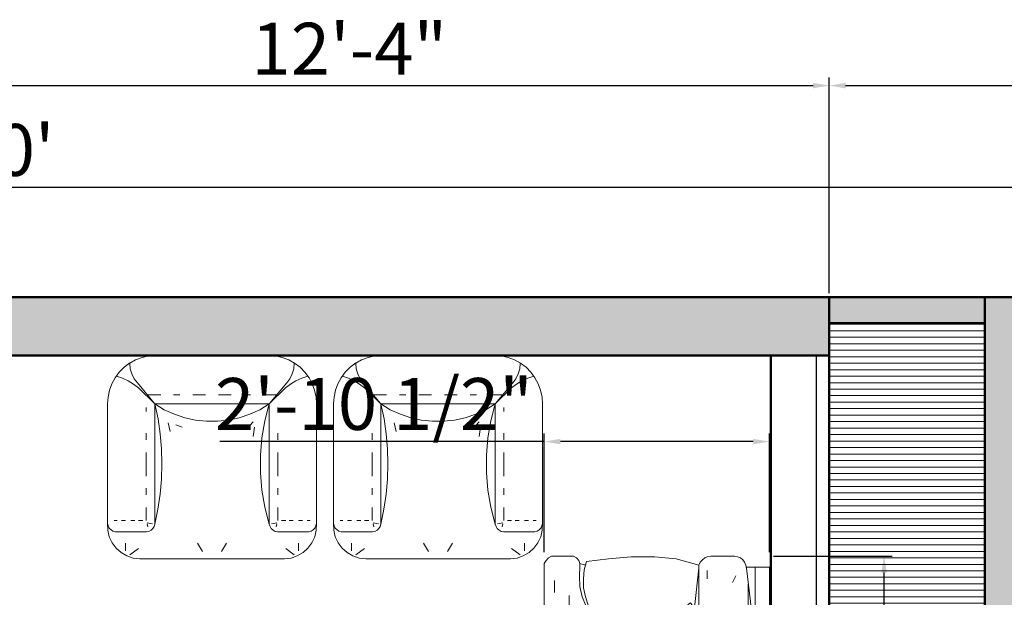
# Model space of a CAD drawing. Units: inches. Extents: x 1770 to 3141, y 984 to 1614.
# Tile 8 of 12: x 2115 to 2267, y 1519 to 1608. Entities that reach past the tile are written whole.
import ezdxf

# ---------------------------------------------------------------- set-up
doc = ezdxf.new("R2010")
doc.units = ezdxf.units.IN
for name, color, linetype, lineweight in [('A-ANNO-DIMS', 2, 'Continuous', 18), ('A-FLOR-PATT', 252, 'Continuous', 13), ('A-FURN', 8, 'Continuous', 18), ('A-GLAZ', 5, 'Continuous', 25), ('A-WALL', 7, 'Continuous', 50), ('A-WALL-PATT', 8, 'Continuous', 13)]:
    doc.layers.add(name, color=color, linetype=linetype, lineweight=lineweight)
doc.styles.get("Standard").update_dxf_attribs({"font": 'arial.ttf'})
doc.dimstyles.new('ISO-25', dxfattribs={"dimtxt": 8, "dimasz": 2.5, "dimexe": 1.25, "dimexo": 0.625, "dimtad": 1, "dimdec": 1, "dimlunit": 3, "dimtxsty": 'Standard', "dimcen": 2.5, "dimclrt": 1, "dimadec": 0, "dimazin": 0, "dimtfac": 1, "dimtdec": 1, "dimtmove": 0, "dimatfit": 3, "dimfxl": 1, "dimarcsym": 0})

# ---------------------------------------------------------------- blocks, each defined once
blk = doc.blocks.new('*D17')
at = {"layer": 'A-ANNO-DIMS', "color": 0, "lineweight": -2, "transparency": 16777216}
for p, q in [((1812.73, 1565.8), (1812.73, 1583.37)), ((2412.73, 1565.8), (2412.73, 1583.37)), ((1815.23, 1582.12), (2410.23, 1582.12))]:
    blk.add_line(p, q, dxfattribs=at)
at = {"layer": 'A-ANNO-DIMS', "color": 0, "transparency": 16777216}
for points in [[(1815.23, 1582.54), (1815.23, 1581.7), (1812.73, 1582.12)], [(2410.23, 1582.54), (2410.23, 1581.7), (2412.73, 1582.12)]]:
    blk.add_solid(points, dxfattribs=at)
at = {"layer": 'Defpoints', "color": 0, "transparency": 16777216}
for p in [(2412.73, 1582.12), (1812.73, 1565.18), (2412.73, 1565.18)]:
    blk.add_point(p, dxfattribs=at)
at = {"layer": 'A-ANNO-DIMS', "color": 0, "transparency": 16777216, "insert": (2112.73, 1586.83), "char_height": 8, "attachment_point": 5}
blk.add_mtext("50'", dxfattribs=at)
blk = doc.blocks.new('sofa-42')
at = {"color": 0, "linetype": 'ByBlock'}
for p, q in [((-0.038, 0.929), (-0.045, 0.917)), ((-0.045, 0.917), (-0.038, 0.929)), ((-0.045, 0.917), (-0.045, 0.824)), ((-0.045, 0.917), (-0.045, 0.824)), ((-0.028, 0.939), (-0.038, 0.929)), ((-0.038, 0.929), (-0.028, 0.939)), ((-0.015, 0.947), (-0.028, 0.939)), ((-0.028, 0.939), (-0.015, 0.947)), ((-0.003, 0.947), (-0.015, 0.947)), ((-0.015, 0.947), (-0.003, 0.947)), ((0.665, 0.947), (-0.003, 0.947)), ((-0.003, 0.947), (0.665, 0.947)), ((0.687, 0.942), (0.665, 0.947)), ((0.687, 0.942), (0.665, 0.947)), ((0.712, 0.932), (0.687, 0.942)), ((0.712, 0.932), (0.687, 0.942)), ((0.73, 0.917), (0.712, 0.932)), ((0.73, 0.917), (0.712, 0.932)), ((0.745, 0.897), (0.73, 0.917)), ((0.745, 0.897), (0.73, 0.917)), ((0.785, 0.917), (0.77, 0.897)), ((0.77, 0.897), (0.785, 0.917)), ((0.802, 0.932), (0.785, 0.917)), ((0.785, 0.917), (0.802, 0.932)), ((0.827, 0.942), (0.802, 0.932)), ((0.802, 0.932), (0.827, 0.942)), ((0.85, 0.947), (0.827, 0.942)), ((0.827, 0.942), (0.85, 0.947)), ((1.462, 0.947), (0.85, 0.947)), ((0.85, 0.947), (1.462, 0.947)), ((1.484, 0.942), (1.462, 0.947)), ((1.484, 0.942), (1.462, 0.947)), ((1.509, 0.932), (1.484, 0.942)), ((1.509, 0.932), (1.484, 0.942)), ((1.527, 0.917), (1.509, 0.932)), ((1.527, 0.917), (1.509, 0.932)), ((1.542, 0.897), (1.527, 0.917)), ((1.542, 0.897), (1.527, 0.917)), ((1.567, 0.897), (1.582, 0.917)), ((1.582, 0.917), (1.567, 0.897)), ((1.582, 0.917), (1.599, 0.932)), ((1.599, 0.932), (1.582, 0.917)), ((1.599, 0.932), (1.624, 0.942)), ((1.624, 0.942), (1.599, 0.932)), ((1.624, 0.942), (1.647, 0.947)), ((1.647, 0.947), (1.624, 0.942)), ((1.647, 0.947), (2.272, 0.947)), ((2.272, 0.947), (1.647, 0.947)), ((2.297, 0.942), (2.272, 0.947)), ((2.297, 0.942), (2.272, 0.947)), ((2.319, 0.932), (2.297, 0.942)), ((2.319, 0.932), (2.297, 0.942)), ((2.337, 0.917), (2.319, 0.932)), ((2.337, 0.917), (2.319, 0.932)), ((2.352, 0.897), (2.337, 0.917)), ((2.352, 0.897), (2.337, 0.917)), ((2.392, 0.917), (2.377, 0.897)), ((2.377, 0.897), (2.392, 0.917)), ((2.412, 0.932), (2.392, 0.917)), ((2.392, 0.917), (2.412, 0.932)), ((2.434, 0.942), (2.412, 0.932)), ((2.412, 0.932), (2.434, 0.942)), ((2.457, 0.947), (2.434, 0.942)), ((2.434, 0.942), (2.457, 0.947)), ((3.127, 0.947), (2.457, 0.947)), ((2.457, 0.947), (3.127, 0.947)), ((3.139, 0.947), (3.127, 0.947)), ((3.139, 0.947), (3.127, 0.947)), ((3.152, 0.939), (3.139, 0.947)), ((3.152, 0.939), (3.139, 0.947)), ((3.162, 0.929), (3.152, 0.939)), ((3.162, 0.929), (3.152, 0.939)), ((3.169, 0.917), (3.162, 0.929)), ((3.169, 0.917), (3.162, 0.929)), ((3.169, 0.824), (3.169, 0.917)), ((3.169, 0.917), (3.169, 0.824)), ((0.042, 0.909), (0.087, 0.889)), ((0.672, 0.892), (0.627, 0.849)), ((0.7, 0.874), (0.685, 0.824)), ((0.755, 0.872), (0.745, 0.897)), ((0.755, 0.872), (0.745, 0.897)), ((0.757, 0.849), (0.755, 0.872)), ((0.757, 0.849), (0.755, 0.872)), ((0.76, 0.872), (0.757, 0.849)), ((0.757, 0.849), (0.76, 0.872)), ((0.77, 0.897), (0.76, 0.872)), ((0.76, 0.872), (0.77, 0.897)), ((0.815, 0.874), (0.83, 0.824)), ((0.842, 0.892), (0.887, 0.849)), ((1.469, 0.892), (1.424, 0.849)), ((1.497, 0.874), (1.482, 0.824)), ((1.552, 0.872), (1.542, 0.897)), ((1.552, 0.872), (1.542, 0.897)), ((1.554, 0.849), (1.552, 0.872)), ((1.554, 0.849), (1.552, 0.872)), ((1.554, 0.849), (1.557, 0.872)), ((1.557, 0.872), (1.554, 0.849)), ((1.557, 0.872), (1.567, 0.897)), ((1.567, 0.897), (1.557, 0.872)), ((1.612, 0.874), (1.627, 0.824)), ((1.639, 0.892), (1.684, 0.849)), ((2.252, 0.887), (2.204, 0.877)), ((2.294, 0.884), (2.257, 0.829)), ((2.362, 0.872), (2.352, 0.897)), ((2.362, 0.872), (2.352, 0.897)), ((2.364, 0.849), (2.362, 0.872)), ((2.364, 0.849), (2.362, 0.872)), ((2.367, 0.872), (2.364, 0.849)), ((2.364, 0.849), (2.367, 0.872)), ((2.377, 0.897), (2.367, 0.872)), ((2.367, 0.872), (2.377, 0.897)), ((2.437, 0.884), (2.474, 0.829)), ((2.477, 0.887), (2.477, 0.877)), ((3.067, 0.904), (3.017, 0.904)), ((0.04, 0.799), (0.037, 0.839)), ((0.757, 0.345), (0.757, 0.849)), ((1.554, 0.06), (1.554, 0.849)), ((2.364, 0.345), (2.364, 0.849)), ((3.004, 0.842), (2.929, 0.842)), ((-0.045, 0.824), (-0.038, 0.812)), ((-0.045, 0.824), (-0.038, 0.812)), ((-0.038, 0.812), (-0.028, 0.802)), ((-0.038, 0.812), (-0.028, 0.802)), ((-0.028, 0.802), (-0.015, 0.797)), ((-0.028, 0.802), (-0.015, 0.797)), ((-0.015, 0.797), (-0.0064, 0.7737)), ((-0.015, 0.797), (-0.003, 0.797)), ((-0.0064, 0.7737), (-0.015, 0.797)), ((0.04, 0.799), (-0.003, 0.797)), ((0.082, 0.797), (0.04, 0.799)), ((0.125, 0.787), (0.082, 0.797)), ((0.162, 0.772), (0.125, 0.787)), ((2.962, 0.772), (2.999, 0.787)), ((2.999, 0.787), (3.042, 0.797)), ((3.042, 0.797), (3.084, 0.799)), ((3.084, 0.799), (3.127, 0.797)), ((3.139, 0.797), (3.127, 0.797)), ((3.1318, 0.7734), (3.139, 0.797)), ((3.1318, 0.7734), (3.139, 0.797)), ((3.139, 0.797), (3.152, 0.802)), ((3.152, 0.802), (3.139, 0.797)), ((3.152, 0.802), (3.162, 0.812)), ((3.162, 0.812), (3.152, 0.802)), ((3.162, 0.812), (3.169, 0.824)), ((3.169, 0.824), (3.162, 0.812)), ((-0.023, 0.769), (-0.035, 0.677)), ((-0.023, 0.769), (-0.035, 0.677)), ((0.012, 0.779), (-0.023, 0.769)), ((-0.0064, 0.7737), (-0.023, 0.769)), ((0.05, 0.782), (0.012, 0.779)), ((0.087, 0.782), (0.05, 0.782)), ((0.125, 0.774), (0.087, 0.782)), ((0.16, 0.762), (0.125, 0.774)), ((0.175, 0.697), (0.16, 0.762)), ((0.177, 0.747), (0.162, 0.772)), ((0.187, 0.719), (0.177, 0.747)), ((2.937, 0.719), (2.947, 0.747)), ((2.947, 0.747), (2.962, 0.772)), ((2.949, 0.697), (2.964, 0.762)), ((2.964, 0.762), (2.999, 0.774)), ((2.999, 0.774), (3.037, 0.782)), ((3.037, 0.782), (3.074, 0.782)), ((3.074, 0.782), (3.112, 0.779)), ((3.112, 0.779), (3.147, 0.769)), ((3.147, 0.769), (3.1318, 0.7734)), ((3.159, 0.677), (3.147, 0.769)), ((3.147, 0.769), (3.159, 0.677)), ((0.192, 0.692), (0.187, 0.719)), ((2.932, 0.692), (2.937, 0.719)), ((-0.035, 0.677), (-0.043, 0.582)), ((-0.035, 0.677), (-0.043, 0.582)), ((0.187, 0.629), (0.175, 0.697)), ((0.202, 0.619), (0.192, 0.692)), ((2.922, 0.619), (2.932, 0.692)), ((2.937, 0.629), (2.949, 0.697)), ((3.167, 0.582), (3.159, 0.677)), ((3.159, 0.677), (3.167, 0.582)), ((0.192, 0.562), (0.187, 0.629)), ((0.267, 0.632), (0.252, 0.607)), ((0.322, 0.599), (0.267, 0.632)), ((2.932, 0.562), (2.937, 0.629)), ((-0.043, 0.582), (-0.043, 0.484)), ((-0.043, 0.582), (-0.043, 0.484)), ((0.207, 0.547), (0.202, 0.619)), ((0.245, 0.594), (0.232, 0.567)), ((0.252, 0.607), (0.245, 0.594)), ((0.332, 0.597), (0.322, 0.599)), ((0.362, 0.584), (0.332, 0.597)), ((0.385, 0.569), (0.362, 0.584)), ((2.732, 0.587), (2.709, 0.572)), ((2.767, 0.617), (2.732, 0.587)), ((2.792, 0.577), (2.767, 0.617)), ((2.917, 0.547), (2.922, 0.619)), ((3.167, 0.484), (3.167, 0.582)), ((3.167, 0.582), (3.167, 0.484)), ((0.195, 0.497), (0.192, 0.562)), ((0.207, 0.492), (0.207, 0.547)), ((0.222, 0.542), (0.215, 0.514)), ((0.232, 0.567), (0.222, 0.542)), ((0.222, 0.542), (0.23, 0.519)), ((0.397, 0.562), (0.385, 0.569)), ((0.405, 0.554), (0.397, 0.562)), ((0.42, 0.534), (0.405, 0.554)), ((0.807, 0.557), (0.8, 0.529)), ((0.87, 0.539), (0.807, 0.557)), ((0.88, 0.542), (0.87, 0.539)), ((0.912, 0.537), (0.88, 0.542)), ((2.702, 0.552), (2.659, 0.514)), ((2.709, 0.572), (2.702, 0.552)), ((2.744, 0.577), (2.712, 0.552)), ((2.764, 0.572), (2.772, 0.532)), ((2.799, 0.567), (2.792, 0.577)), ((2.819, 0.542), (2.799, 0.567)), ((2.844, 0.507), (2.819, 0.542)), ((2.917, 0.474), (2.917, 0.547)), ((2.929, 0.497), (2.932, 0.562)), ((0.195, 0.482), (0.195, 0.497)), ((0.215, 0.514), (0.212, 0.487)), ((0.23, 0.519), (0.23, 0.497)), ((0.23, 0.497), (0.23, 0.477)), ((0.425, 0.537), (0.42, 0.534)), ((0.46, 0.524), (0.425, 0.537)), ((0.467, 0.512), (0.46, 0.524)), ((0.475, 0.507), (0.467, 0.512)), ((0.492, 0.492), (0.475, 0.507)), ((0.797, 0.517), (0.792, 0.484)), ((0.8, 0.529), (0.797, 0.517)), ((0.937, 0.529), (0.912, 0.537)), ((0.952, 0.524), (0.937, 0.529)), ((0.962, 0.519), (0.952, 0.524)), ((0.982, 0.502), (0.962, 0.519)), ((0.987, 0.507), (0.982, 0.502)), ((1.022, 0.502), (0.987, 0.507)), ((1.035, 0.492), (1.022, 0.502)), ((2.632, 0.499), (2.624, 0.487)), ((2.659, 0.514), (2.632, 0.499)), ((2.637, 0.504), (2.642, 0.502)), ((2.867, 0.47), (2.844, 0.507)), ((2.932, 0.43), (2.929, 0.497)), ((-0.043, 0.484), (-0.035, 0.392)), ((-0.043, 0.484), (-0.035, 0.392)), ((0.185, 0.462), (0.177, 0.43)), ((0.192, 0.472), (0.185, 0.462)), ((0.212, 0.487), (0.192, 0.472)), ((0.207, 0.467), (0.212, 0.487)), ((0.207, 0.452), (0.207, 0.467)), ((0.507, 0.484), (0.492, 0.492)), ((0.522, 0.479), (0.507, 0.484)), ((0.532, 0.482), (0.522, 0.479)), ((0.552, 0.467), (0.532, 0.482)), ((0.57, 0.457), (0.552, 0.467)), ((0.572, 0.452), (0.57, 0.457)), ((0.79, 0.462), (0.787, 0.432)), ((0.792, 0.484), (0.79, 0.462)), ((0.79, 0.462), (0.802, 0.442)), ((1.042, 0.492), (1.035, 0.492)), ((1.062, 0.482), (1.042, 0.492)), ((1.074, 0.477), (1.062, 0.482)), ((1.092, 0.477), (1.074, 0.477)), ((1.102, 0.482), (1.092, 0.477)), ((1.124, 0.472), (1.102, 0.482)), ((1.144, 0.467), (1.124, 0.472)), ((1.134, 0.427), (1.147, 0.465)), ((1.147, 0.465), (1.144, 0.467)), ((2.572, 0.457), (2.547, 0.447)), ((2.599, 0.467), (2.572, 0.457)), ((2.572, 0.457), (2.617, 0.45)), ((2.624, 0.487), (2.599, 0.467)), ((2.599, 0.467), (2.612, 0.47)), ((2.612, 0.47), (2.637, 0.467)), ((2.872, 0.422), (2.859, 0.479)), ((2.912, 0.427), (2.867, 0.47)), ((2.922, 0.405), (2.917, 0.474)), ((3.159, 0.392), (3.167, 0.484)), ((3.167, 0.484), (3.159, 0.392)), ((0.177, 0.43), (0.145, 0.395)), ((0.277, 0.425), (0.265, 0.432)), ((0.307, 0.407), (0.277, 0.425)), ((0.532, 0.407), (0.55, 0.422)), ((0.55, 0.422), (0.572, 0.452)), ((0.787, 0.432), (0.792, 0.407)), ((0.802, 0.442), (0.807, 0.42)), ((0.807, 0.42), (0.812, 0.4)), ((1.122, 0.41), (1.134, 0.427)), ((2.514, 0.437), (2.479, 0.417)), ((2.479, 0.417), (2.479, 0.412)), ((2.534, 0.442), (2.514, 0.437)), ((2.547, 0.447), (2.534, 0.442)), ((2.617, 0.45), (2.629, 0.452)), ((2.879, 0.377), (2.832, 0.432)), ((2.929, 0.382), (2.912, 0.427)), ((2.937, 0.362), (2.932, 0.43)), ((-0.035, 0.392), (-0.02, 0.292)), ((-0.035, 0.392), (-0.02, 0.292)), ((0.112, 0.34), (0.145, 0.38)), ((0.145, 0.395), (0.117, 0.367)), ((0.237, 0.397), (0.315, 0.385)), ((0.337, 0.405), (0.307, 0.407)), ((0.315, 0.385), (0.352, 0.375)), ((0.377, 0.387), (0.337, 0.405)), ((0.352, 0.375), (0.377, 0.387)), ((0.377, 0.387), (0.417, 0.392)), ((0.505, 0.377), (0.462, 0.367)), ((0.485, 0.357), (0.505, 0.377)), ((0.505, 0.377), (0.525, 0.397)), ((0.525, 0.397), (0.532, 0.407)), ((0.777, 0.385), (0.772, 0.372)), ((0.792, 0.407), (0.777, 0.385)), ((0.795, 0.382), (0.792, 0.407)), ((0.797, 0.37), (0.795, 0.382)), ((1.102, 0.375), (1.062, 0.352)), ((1.087, 0.347), (1.102, 0.375)), ((1.102, 0.375), (1.117, 0.4)), ((1.117, 0.4), (1.122, 0.41)), ((2.479, 0.412), (2.492, 0.395)), ((2.492, 0.395), (2.502, 0.372)), ((2.684, 0.397), (2.647, 0.407)), ((2.684, 0.397), (2.712, 0.362)), ((2.714, 0.397), (2.684, 0.397)), ((2.742, 0.372), (2.714, 0.397)), ((2.927, 0.375), (2.922, 0.405)), ((2.927, 0.37), (2.929, 0.382)), ((3.132, 0.297), (3.159, 0.392)), ((3.159, 0.392), (3.132, 0.297)), ((0.117, 0.367), (0.087, 0.322)), ((0.132, 0.335), (0.177, 0.337)), ((0.462, 0.367), (0.452, 0.36)), ((0.477, 0.35), (0.452, 0.342)), ((0.472, 0.327), (0.485, 0.357)), ((0.607, 0.34), (0.475, 0.335)), ((0.485, 0.357), (0.477, 0.35)), ((0.775, 0.34), (0.607, 0.34)), ((0.775, 0.34), (0.752, 0.297)), ((0.752, 0.297), (0.752, 0.34)), ((0.772, 0.372), (0.775, 0.34)), ((0.872, 0.36), (0.857, 0.362)), ((0.905, 0.35), (0.872, 0.36)), ((0.935, 0.357), (0.905, 0.35)), ((0.98, 0.347), (0.935, 0.357)), ((0.957, 0.33), (0.98, 0.347)), ((0.98, 0.347), (1.017, 0.365)), ((1.062, 0.352), (1.057, 0.342)), ((1.082, 0.34), (1.059, 0.327)), ((1.087, 0.347), (1.082, 0.34)), ((1.082, 0.317), (1.087, 0.347)), ((2.219, 0.347), (1.087, 0.347)), ((2.422, 0.34), (2.219, 0.347)), ((2.372, 0.06), (2.372, 0.34)), ((2.542, 0.332), (2.422, 0.34)), ((2.502, 0.372), (2.512, 0.372)), ((2.512, 0.372), (2.524, 0.36)), ((2.524, 0.36), (2.534, 0.347)), ((2.534, 0.347), (2.544, 0.325)), ((2.712, 0.362), (2.739, 0.347)), ((2.739, 0.347), (2.759, 0.317)), ((2.807, 0.325), (2.742, 0.372)), ((2.929, 0.34), (2.887, 0.357)), ((2.934, 0.36), (2.927, 0.37)), ((2.929, 0.302), (2.974, 0.332)), ((2.967, 0.342), (2.934, 0.36)), ((2.939, 0.357), (2.937, 0.362)), ((2.974, 0.332), (2.967, 0.342)), ((-0.02, 0.292), (-0.03, 0.282)), ((-0.02, 0.292), (-0.03, 0.282)), ((-0.008, 0.297), (-0.02, 0.292)), ((0.14, 0.312), (-0.008, 0.297)), ((-0.008, 0.297), (0.15, 0.297)), ((0.005, 0.297), (-0.008, 0.297)), ((0.087, 0.322), (0.1, 0.317)), ((0.1, 0.317), (0.135, 0.315)), ((0.135, 0.315), (0.147, 0.307)), ((0.147, 0.307), (0.152, 0.295)), ((0.152, 0.295), (0.185, 0.262)), ((0.452, 0.287), (0.47, 0.312)), ((0.46, 0.297), (0.752, 0.297)), ((0.467, 0.307), (0.462, 0.307)), ((0.47, 0.312), (0.472, 0.327)), ((0.752, 0.297), (0.732, 0.262)), ((0.84, 0.325), (0.917, 0.33)), ((0.917, 0.33), (0.957, 0.33)), ((1.074, 0.272), (1.087, 0.302)), ((1.084, 0.297), (1.079, 0.292)), ((1.087, 0.302), (1.082, 0.317)), ((1.0855, 0.2985), (1.084, 0.297)), ((1.084, 0.297), (1.0848, 0.297)), ((1.084, 0.297), (2.372, 0.297)), ((1.0848, 0.297), (1.0855, 0.2985)), ((2.372, 0.297), (2.557, 0.297)), ((2.544, 0.325), (2.547, 0.32)), ((2.547, 0.32), (2.552, 0.302)), ((2.552, 0.302), (2.577, 0.28)), ((2.759, 0.317), (2.767, 0.307)), ((2.847, 0.272), (2.892, 0.29)), ((2.892, 0.29), (2.929, 0.302)), ((2.944, 0.327), (2.899, 0.305)), ((2.914, 0.297), (3.119, 0.297)), ((2.927, 0.317), (2.924, 0.317)), ((2.954, 0.315), (2.947, 0.317)), ((2.947, 0.315), (2.947, 0.317)), ((3.119, 0.297), (2.954, 0.315)), ((3.132, 0.297), (3.119, 0.297)), ((3.144, 0.292), (3.132, 0.297)), ((3.144, 0.292), (3.132, 0.297)), ((3.154, 0.282), (3.144, 0.292)), ((3.154, 0.282), (3.144, 0.292)), ((-0.043, 0.262), (-0.045, 0.247)), ((-0.043, 0.262), (-0.045, 0.247)), ((-0.038, 0.272), (-0.043, 0.262)), ((-0.038, 0.272), (-0.043, 0.262)), ((-0.03, 0.282), (-0.038, 0.272)), ((-0.03, 0.282), (-0.038, 0.272)), ((-0.005, 0.262), (0.007, 0.25)), ((0.185, 0.262), (0.242, 0.242)), ((0.43, 0.235), (0.452, 0.287)), ((0.732, 0.262), (0.715, 0.212)), ((0.737, 0.237), (0.755, 0.282)), ((0.755, 0.237), (0.797, 0.25)), ((1.067, 0.217), (1.074, 0.272)), ((2.577, 0.28), (2.582, 0.28)), ((2.582, 0.28), (2.587, 0.252)), ((2.587, 0.252), (2.592, 0.242)), ((2.769, 0.23), (2.779, 0.25)), ((2.804, 0.25), (2.792, 0.232)), ((2.809, 0.262), (2.804, 0.25)), ((2.827, 0.245), (2.847, 0.272)), ((3.109, 0.262), (3.074, 0.262)), ((3.162, 0.272), (3.154, 0.282)), ((3.162, 0.272), (3.154, 0.282)), ((3.167, 0.262), (3.162, 0.272)), ((3.167, 0.262), (3.162, 0.272)), ((3.169, 0.247), (3.167, 0.262)), ((3.169, 0.247), (3.167, 0.262)), ((-0.045, 0.247), (-0.045, 0.147)), ((-0.045, 0.247), (-0.045, 0.147)), ((0.242, 0.242), (0.28, 0.215)), ((0.28, 0.215), (0.317, 0.195)), ((0.38, 0.192), (0.355, 0.225)), ((0.4, 0.197), (0.42, 0.232)), ((0.415, 0.19), (0.43, 0.215)), ((0.43, 0.215), (0.43, 0.235)), ((0.715, 0.212), (0.727, 0.21)), ((0.727, 0.21), (0.765, 0.217)), ((0.752, 0.06), (0.752, 0.215)), ((0.765, 0.217), (0.777, 0.215)), ((0.777, 0.215), (0.785, 0.202)), ((1.05, 0.172), (1.057, 0.212)), ((1.072, 0.197), (1.067, 0.217)), ((2.592, 0.242), (2.599, 0.23)), ((2.599, 0.23), (2.614, 0.207)), ((2.757, 0.187), (2.762, 0.212)), ((2.757, 0.187), (2.777, 0.21)), ((2.762, 0.212), (2.769, 0.23)), ((2.777, 0.21), (2.792, 0.232)), ((2.792, 0.232), (2.817, 0.237)), ((2.817, 0.237), (2.827, 0.245)), ((3.169, 0.147), (3.169, 0.247)), ((3.169, 0.147), (3.169, 0.247)), ((0.317, 0.195), (0.347, 0.182)), ((0.347, 0.182), (0.357, 0.175)), ((0.357, 0.175), (0.397, 0.147)), ((0.397, 0.147), (0.415, 0.19)), ((0.785, 0.202), (0.827, 0.18)), ((0.827, 0.18), (0.887, 0.175)), ((0.887, 0.175), (0.93, 0.16)), ((1.032, 0.162), (1, 0.187)), ((1.057, 0.125), (1.064, 0.17)), ((1.064, 0.17), (1.072, 0.197)), ((2.614, 0.207), (2.637, 0.182)), ((2.637, 0.182), (2.644, 0.177)), ((2.644, 0.177), (2.682, 0.125)), ((2.717, 0.15), (2.739, 0.17)), ((2.739, 0.17), (2.757, 0.187)), ((-0.045, 0.147), (-0.043, 0.135)), ((-0.045, 0.147), (-0.043, 0.135)), ((-0.043, 0.135), (-0.038, 0.122)), ((-0.043, 0.135), (-0.038, 0.122)), ((-0.008, 0.132), (0.02, 0.142)), ((0.93, 0.16), (0.97, 0.147)), ((0.97, 0.147), (1.002, 0.142)), ((1.002, 0.142), (1.015, 0.14)), ((1.015, 0.14), (1.057, 0.125)), ((2.682, 0.125), (2.704, 0.142)), ((2.704, 0.142), (2.717, 0.15)), ((3.087, 0.142), (3.059, 0.155)), ((3.162, 0.122), (3.167, 0.135)), ((3.162, 0.122), (3.167, 0.135)), ((3.167, 0.135), (3.169, 0.147)), ((3.167, 0.135), (3.169, 0.147)), ((-0.038, 0.122), (-0.03, 0.112)), ((-0.038, 0.122), (-0.03, 0.112)), ((-0.03, 0.112), (-0.02, 0.105)), ((-0.03, 0.112), (-0.02, 0.105)), ((-0.02, 0.105), (-0.008, 0.1)), ((-0.02, 0.105), (-0.008, 0.1)), ((-0.008, 0.1), (0, 0.0982)), ((-0.008, 0.1), (0.005, 0.097)), ((0, 0.1), (0, 0)), ((0, 0.0982), (0, 0)), ((0.005, 0.097), (0.145, 0.08)), ((0.072, 0.09), (0.752, 0.09)), ((0.752, 0.09), (2.372, 0.09)), ((2.372, 0.09), (3.052, 0.09)), ((2.979, 0.08), (3.119, 0.097)), ((3.119, 0.097), (3.132, 0.1)), ((3.124, 0.0982), (3.132, 0.1)), ((3.124, 0.1), (3.124, 0)), ((3.124, 0), (3.124, 0.0982)), ((3.132, 0.1), (3.144, 0.105)), ((3.132, 0.1), (3.144, 0.105)), ((3.144, 0.105), (3.154, 0.112)), ((3.144, 0.105), (3.154, 0.112)), ((3.154, 0.112), (3.162, 0.122)), ((3.154, 0.112), (3.162, 0.122)), ((0.145, 0.08), (0.285, 0.067)), ((0.285, 0.067), (0.425, 0.06)), ((0.425, 0.06), (3.124, 0.06)), ((2.699, 0.06), (2.839, 0.067)), ((2.839, 0.067), (2.979, 0.08)), ((0, 0), (3.124, 0)), ((0, 0), (3.124, 0))]:
    blk.add_line(p, q, dxfattribs=at)
blk = doc.blocks.new('sofa-47')
at = {"color": 0, "linetype": 'ByBlock'}
for p, q in [((-0.1206, 0.8424), (-0.1449, 0.828)), ((-0.1206, 0.8424), (-0.1449, 0.828)), ((-0.0945, 0.8514), (-0.1206, 0.8424)), ((-0.0945, 0.8514), (-0.1206, 0.8424)), ((-0.072, 0.8109), (-0.108, 0.8379)), ((-0.0666, 0.855), (-0.0945, 0.8514)), ((-0.0666, 0.855), (-0.0945, 0.8514)), ((0.2376, 0.855), (-0.0666, 0.855)), ((0.2376, 0.855), (-0.0666, 0.855)), ((0.5418, 0.855), (0.2376, 0.855)), ((0.5418, 0.855), (0.2376, 0.855)), ((0.5697, 0.8514), (0.5418, 0.855)), ((0.5697, 0.8514), (0.5418, 0.855)), ((0.5472, 0.8109), (0.5832, 0.8379)), ((0.5958, 0.8424), (0.5697, 0.8514)), ((0.5958, 0.8424), (0.5697, 0.8514)), ((0.6201, 0.828), (0.5958, 0.8424)), ((0.6201, 0.828), (0.5958, 0.8424)), ((-0.1827, 0.7875), (-0.1944, 0.7614)), ((-0.1827, 0.7875), (-0.1944, 0.7614)), ((-0.1656, 0.81), (-0.1827, 0.7875)), ((-0.1656, 0.81), (-0.1827, 0.7875)), ((-0.1449, 0.828), (-0.1656, 0.81)), ((-0.1449, 0.828), (-0.1656, 0.81)), ((-0.126, 0.8208), (-0.126, 0.7884)), ((0.1764, 0.7884), (0.198, 0.8235)), ((0.2772, 0.8235), (0.2988, 0.7884)), ((0.6012, 0.8208), (0.6012, 0.7884)), ((0.6408, 0.81), (0.6201, 0.828)), ((0.6408, 0.81), (0.6201, 0.828)), ((0.6579, 0.7875), (0.6408, 0.81)), ((0.6579, 0.7875), (0.6408, 0.81)), ((0.6696, 0.7614), (0.6579, 0.7875)), ((0.6696, 0.7614), (0.6579, 0.7875)), ((-0.1944, 0.7614), (-0.2007, 0.7344)), ((-0.1944, 0.7614), (-0.2007, 0.7344)), ((0.6759, 0.7344), (0.6696, 0.7614)), ((0.6759, 0.7344), (0.6696, 0.7614)), ((-0.2007, 0.7344), (-0.2016, 0.7065)), ((-0.2007, 0.7344), (-0.2016, 0.7065)), ((-0.2016, 0.7065), (-0.1989, 0.7164)), ((-0.2016, 0.7065), (-0.2016, 0.2034)), ((-0.2016, 0.2034), (-0.2016, 0.7065)), ((-0.1989, 0.7164), (-0.1944, 0.7254)), ((-0.1944, 0.7254), (-0.1872, 0.7326)), ((-0.1872, 0.7326), (-0.1791, 0.738)), ((-0.1791, 0.738), (-0.1692, 0.7407)), ((-0.1692, 0.7407), (-0.1593, 0.7416)), ((-0.1593, 0.7416), (-0.0486, 0.7416)), ((-0.0486, 0.7416), (-0.0378, 0.7416)), ((-0.0378, 0.7416), (-0.0279, 0.7389)), ((-0.0351, 0.7074), (-0.0324, 0.72)), ((-0.0351, 0.7029), (-0.0126, 0.7074)), ((-0.0279, 0.7389), (-0.0189, 0.7335)), ((-0.0189, 0.7335), (-0.0117, 0.7263)), ((-0.0117, 0.7263), (-0.0063, 0.7182)), ((-0.0063, 0.7182), (-0.0027, 0.7083)), ((0.0099, 0.6462), (-0.0027, 0.7083)), ((-0.0027, 0.7083), (-0.0027, 0.6975)), ((0.4779, 0.7083), (0.4599, 0.6372)), ((0.4779, 0.7083), (0.4815, 0.7182)), ((0.4779, 0.6975), (0.4779, 0.7083)), ((0.4815, 0.7182), (0.4869, 0.7263)), ((0.4869, 0.7263), (0.4941, 0.7335)), ((0.5103, 0.7029), (0.4878, 0.7074)), ((0.4941, 0.7335), (0.5031, 0.7389)), ((0.5031, 0.7389), (0.513, 0.7416)), ((0.5103, 0.7074), (0.5076, 0.72)), ((0.513, 0.7416), (0.5238, 0.7416)), ((0.5238, 0.7416), (0.6345, 0.7416)), ((0.6345, 0.7416), (0.6444, 0.7407)), ((0.6444, 0.7407), (0.6543, 0.738)), ((0.6543, 0.738), (0.6624, 0.7326)), ((0.6624, 0.7326), (0.6696, 0.7254)), ((0.6696, 0.7254), (0.6741, 0.7164)), ((0.6741, 0.7164), (0.6768, 0.7065)), ((0.6768, 0.7065), (0.6759, 0.7344)), ((0.6768, 0.7065), (0.6759, 0.7344)), ((0.6768, 0.2034), (0.6768, 0.7065)), ((0.6768, 0.7065), (0.6768, 0.2034)), ((-0.1746, 0.693), (-0.162, 0.693)), ((-0.1431, 0.693), (-0.126, 0.693)), ((-0.1035, 0.693), (-0.0864, 0.693)), ((-0.072, 0.693), (-0.054, 0.693)), ((-0.0396, 0.693), (-0.0396, 0.639)), ((-0.0027, 0.6975), (-0.0027, 0.2034)), ((0.4779, 0.2034), (0.4779, 0.6975)), ((0.5148, 0.693), (0.5148, 0.639)), ((0.5472, 0.693), (0.5292, 0.693)), ((0.5787, 0.693), (0.5616, 0.693)), ((0.6183, 0.693), (0.6012, 0.693)), ((0.6498, 0.693), (0.6372, 0.693)), ((0.0198, 0.5832), (0.0099, 0.6462)), ((0.4599, 0.6372), (0.4473, 0.5652)), ((-0.0396, 0.585), (-0.0396, 0.558)), ((0.0252, 0.5193), (0.0198, 0.5832)), ((0.5148, 0.585), (0.5148, 0.558)), ((0.4473, 0.5652), (0.441, 0.4923)), ((-0.0396, 0.4077), (-0.0396, 0.5067)), ((0.027, 0.4554), (0.0252, 0.5193)), ((0.5148, 0.4077), (0.5148, 0.5067)), ((0.441, 0.4923), (0.441, 0.4194)), ((0.0252, 0.3924), (0.027, 0.4554)), ((0.441, 0.4194), (0.4473, 0.3465)), ((0.0198, 0.3285), (0.0252, 0.3924)), ((-0.0396, 0.3267), (-0.0396, 0.3537)), ((0.4167, 0.3015), (0.4104, 0.3402)), ((0.4473, 0.3465), (0.4599, 0.2745)), ((0.5148, 0.3267), (0.5148, 0.3537)), ((0.0108, 0.2655), (0.0198, 0.3285)), ((0.0531, 0.2826), (0.0621, 0.3186)), ((0.0855, 0.2907), (0.1116, 0.3015)), ((0.4104, 0.2781), (0.3969, 0.2934)), ((-0.0027, 0.2034), (0.0108, 0.2655)), ((0.1233, 0.2619), (0.0792, 0.2466)), ((0.1683, 0.2718), (0.1233, 0.2619)), ((0.2142, 0.2763), (0.1683, 0.2718)), ((0.261, 0.2763), (0.2142, 0.2763)), ((0.3069, 0.2718), (0.261, 0.2763)), ((0.3519, 0.2619), (0.3069, 0.2718)), ((0.396, 0.2466), (0.3519, 0.2619)), ((0.4599, 0.2745), (0.4779, 0.2034)), ((-0.0396, 0.2187), (-0.0396, 0.2358)), ((0.0369, 0.2277), (-0.0027, 0.2034)), ((0.0792, 0.2466), (0.0369, 0.2277)), ((0.4383, 0.2277), (0.396, 0.2466)), ((0.4779, 0.2034), (0.4383, 0.2277)), ((0.5148, 0.2187), (0.5148, 0.2358)), ((-0.2016, 0.2034), (-0.1998, 0.1746)), ((-0.1998, 0.1746), (-0.2016, 0.2034)), ((-0.1998, 0.1746), (-0.1935, 0.1458)), ((-0.1935, 0.1458), (-0.1998, 0.1746)), ((-0.0765, 0.1152), (-0.0045, 0.2016)), ((-0.0045, 0.2016), (-0.0711, 0.135)), ((-0.0027, 0.2034), (0.2376, 0.2034)), ((0.2376, 0.2034), (0.4779, 0.2034)), ((0.4797, 0.2016), (0.5517, 0.1152)), ((0.5463, 0.135), (0.4797, 0.2016)), ((0.6687, 0.1458), (0.675, 0.1746)), ((0.675, 0.1746), (0.6687, 0.1458)), ((0.675, 0.1746), (0.6768, 0.2034)), ((0.6768, 0.2034), (0.675, 0.1746)), ((-0.1935, 0.1458), (-0.1836, 0.1188)), ((-0.1836, 0.1188), (-0.1935, 0.1458)), ((-0.0711, 0.135), (-0.0927, 0.1197)), ((-0.0324, 0.1647), (0.0216, 0.1647)), ((0.0756, 0.1647), (0.1026, 0.1647)), ((0.1566, 0.1647), (0.2106, 0.1647)), ((0.3186, 0.1647), (0.2646, 0.1647)), ((0.3996, 0.1647), (0.3726, 0.1647)), ((0.5076, 0.1647), (0.4536, 0.1647)), ((0.5679, 0.1197), (0.5463, 0.135)), ((0.6588, 0.1188), (0.6687, 0.1458)), ((0.6687, 0.1458), (0.6588, 0.1188)), ((-0.1836, 0.1188), (-0.1701, 0.0936)), ((-0.1701, 0.0936), (-0.1836, 0.1188)), ((-0.1701, 0.0936), (-0.153, 0.0702)), ((-0.153, 0.0702), (-0.1701, 0.0936)), ((-0.1395, 0.0954), (-0.1647, 0.0873)), ((-0.1152, 0.1062), (-0.1395, 0.0954)), ((-0.0927, 0.1197), (-0.1152, 0.1062)), ((-0.0999, 0.0774), (-0.09, 0.0972)), ((-0.09, 0.0972), (-0.0765, 0.1152)), ((0.5517, 0.1152), (0.5652, 0.0972)), ((0.5652, 0.0972), (0.5751, 0.0774)), ((0.5904, 0.1062), (0.5679, 0.1197)), ((0.6147, 0.0954), (0.5904, 0.1062)), ((0.6399, 0.0873), (0.6147, 0.0954)), ((0.6282, 0.0702), (0.6453, 0.0936)), ((0.6453, 0.0936), (0.6282, 0.0702)), ((0.6453, 0.0936), (0.6588, 0.1188)), ((0.6588, 0.1188), (0.6453, 0.0936)), ((-0.153, 0.0702), (-0.1323, 0.0495)), ((-0.1323, 0.0495), (-0.153, 0.0702)), ((-0.1323, 0.0495), (-0.1082, 0.0312)), ((-0.1098, 0.0324), (-0.1323, 0.0495)), ((-0.108, 0.0333), (-0.1062, 0.0558)), ((-0.1062, 0.0558), (-0.0999, 0.0774)), ((0.5751, 0.0774), (0.5814, 0.0558)), ((0.5814, 0.0558), (0.5832, 0.0333)), ((0.585, 0.0324), (0.6075, 0.0495)), ((0.6075, 0.0495), (0.585, 0.0324)), ((0.6075, 0.0495), (0.6282, 0.0702)), ((0.6282, 0.0702), (0.6075, 0.0495)), ((-0.0846, 0.018), (-0.1098, 0.0324)), ((-0.1082, 0.0312), (-0.1081, 0.0315)), ((-0.1081, 0.0315), (-0.0846, 0.018)), ((-0.0846, 0.018), (-0.0567, 0.0081)), ((-0.0567, 0.0081), (-0.0846, 0.018)), ((-0.0567, 0.0081), (-0.0288, 0.0018)), ((-0.0288, 0.0018), (-0.0567, 0.0081)), ((-0.0288, 0.0018), (0, 0)), ((0, 0), (-0.0288, 0.0018)), ((0, 0), (0.2376, 0)), ((0.2376, 0), (0, 0)), ((0.2376, 0), (0.4752, 0)), ((0.4752, 0), (0.2376, 0)), ((0.4752, 0), (0.504, 0.0018)), ((0.504, 0.0018), (0.4752, 0)), ((0.504, 0.0018), (0.5319, 0.0081)), ((0.5319, 0.0081), (0.504, 0.0018)), ((0.5319, 0.0081), (0.5598, 0.018)), ((0.5598, 0.018), (0.5319, 0.0081)), ((0.5598, 0.018), (0.585, 0.0324)), ((0.585, 0.0324), (0.5598, 0.018))]:
    blk.add_line(p, q, dxfattribs=at)
blk = doc.blocks.new('*D88')
at = {"layer": 'A-ANNO-DIMS', "color": 0, "lineweight": -2, "transparency": 16777216}
for p, q in [((2231.13, 1525.24), (2249.43, 1525.24)), ((2248.18, 1409.9), (2248.18, 1522.74)), ((2231.13, 1407.4), (2249.43, 1407.4))]:
    blk.add_line(p, q, dxfattribs=at)
at = {"layer": 'A-ANNO-DIMS', "color": 0, "transparency": 16777216}
for points in [[(2247.77, 1522.74), (2248.6, 1522.74), (2248.18, 1525.24)], [(2247.77, 1409.9), (2248.6, 1409.9), (2248.18, 1407.4)]]:
    blk.add_solid(points, dxfattribs=at)
at = {"layer": 'Defpoints', "color": 0, "transparency": 16777216}
for p in [(2230.51, 1525.24), (2248.18, 1525.24), (2230.51, 1407.4)]:
    blk.add_point(p, dxfattribs=at)
at = {"layer": 'A-ANNO-DIMS', "color": 1, "transparency": 16777216, "insert": (2243.42, 1466.32), "char_height": 8, "attachment_point": 5, "rotation": 90}
blk.add_mtext('SOFA 9\'-10"', dxfattribs=at)
blk = doc.blocks.new('*D89')
at = {"layer": 'A-ANNO-DIMS', "color": 0, "lineweight": -2, "transparency": 16777216}
for p, q in [((2195.79, 1525.87), (2195.79, 1544.17)), ((2230.51, 1525.87), (2230.51, 1544.17)), ((2195.79, 1542.92), (2145.78, 1542.92)), ((2228.01, 1542.92), (2198.29, 1542.92))]:
    blk.add_line(p, q, dxfattribs=at)
at = {"layer": 'A-ANNO-DIMS', "color": 0, "transparency": 16777216}
for points in [[(2198.29, 1543.34), (2198.29, 1542.5), (2195.79, 1542.92)], [(2228.01, 1543.34), (2228.01, 1542.5), (2230.51, 1542.92)]]:
    blk.add_solid(points, dxfattribs=at)
at = {"layer": 'Defpoints', "color": 0, "transparency": 16777216}
for p in [(2195.79, 1542.92), (2195.79, 1525.24), (2230.51, 1525.24)]:
    blk.add_point(p, dxfattribs=at)
at = {"layer": 'A-ANNO-DIMS', "color": 1, "transparency": 16777216, "insert": (2169.53, 1547.68), "char_height": 8, "attachment_point": 5}
blk.add_mtext('2\'-10 1/2"', dxfattribs=at)
blk = doc.blocks.new('*D103')
at = {"layer": 'A-ANNO-DIMS', "color": 0, "lineweight": -2, "transparency": 16777216}
for p, q in [((2091.73, 1556.8), (2091.73, 1599.03)), ((2239.73, 1565.8), (2239.73, 1599.03)), ((2094.23, 1597.78), (2237.23, 1597.78))]:
    blk.add_line(p, q, dxfattribs=at)
at = {"layer": 'A-ANNO-DIMS', "color": 0, "transparency": 16777216}
for points in [[(2094.23, 1598.2), (2094.23, 1597.36), (2091.73, 1597.78)], [(2237.23, 1598.2), (2237.23, 1597.36), (2239.73, 1597.78)]]:
    blk.add_solid(points, dxfattribs=at)
at = {"layer": 'Defpoints', "color": 0, "transparency": 16777216}
for p in [(2239.73, 1597.78), (2239.73, 1565.18), (2091.73, 1556.18)]:
    blk.add_point(p, dxfattribs=at)
at = {"layer": 'A-ANNO-DIMS', "color": 1, "transparency": 16777216, "insert": (2165.73, 1602.42), "char_height": 8, "attachment_point": 5}
blk.add_mtext('12\'-4"', dxfattribs=at)
blk = doc.blocks.new('*D104')
at = {"layer": 'A-ANNO-DIMS', "color": 0, "lineweight": -2, "transparency": 16777216}
for p, q in [((2239.73, 1565.8), (2239.73, 1599.03)), ((2412.73, 1565.8), (2412.73, 1599.03)), ((2242.23, 1597.78), (2410.23, 1597.78))]:
    blk.add_line(p, q, dxfattribs=at)
at = {"layer": 'A-ANNO-DIMS', "color": 0, "transparency": 16777216}
for points in [[(2242.23, 1598.2), (2242.23, 1597.36), (2239.73, 1597.78)], [(2410.23, 1598.2), (2410.23, 1597.36), (2412.73, 1597.78)]]:
    blk.add_solid(points, dxfattribs=at)
at = {"layer": 'Defpoints', "color": 0, "transparency": 16777216}
for p in [(2412.73, 1597.78), (2239.73, 1565.18), (2412.73, 1565.18)]:
    blk.add_point(p, dxfattribs=at)
at = {"layer": 'A-ANNO-DIMS', "color": 1, "transparency": 16777216, "insert": (2326.23, 1602.49), "char_height": 8, "attachment_point": 5}
blk.add_mtext('14\'-5"', dxfattribs=at)

msp = doc.modelspace()

# ---------------------------------------------------------------- hatches: boundary and pattern name
at = {"layer": 'A-FLOR-PATT'}
h = msp.add_hatch(color=256, dxfattribs=at)
h.dxf.hatch_style = 1
h.paths.add_polyline_path([(2263.73, 1565.18), (2239.73, 1565.18), (2239.73, 1561.18), (2263.73, 1561.18)])
h.paths.add_polyline_path([(2412.73, 1565.18), (2384.73, 1565.18), (2384.73, 1561.18), (2408.73, 1561.18), (2408.73, 1300.18), (2412.73, 1300.18)])
h = msp.add_hatch(color=256, dxfattribs=at)
h.dxf.hatch_style = 1
h.paths.add_polyline_path([(2384.73, 1565.18), (2263.73, 1565.18), (2263.73, 1347.18), (2333.73, 1347.18), (2333.73, 1356.18), (2272.73, 1356.18), (2272.73, 1556.18), (2375.73, 1556.18), (2375.73, 1347.18), (2384.73, 1347.18)])
h = msp.add_hatch(dxfattribs=at)
h.set_pattern_fill('_USER', color=256, pattern_type=0)
h.set_pattern_definition([(0, (0, 0), (0, 1), [])])
h.paths.add_polyline_path([(2408.73, 1561.18), (2384.73, 1561.18), (2384.73, 1347.18), (2375.73, 1347.18), (2263.73, 1347.18), (2263.73, 1561.18), (2239.73, 1561.18), (2239.73, 1300.18), (2408.73, 1300.18)])
at = {"layer": 'A-WALL-PATT'}
h = msp.add_hatch(color=256, dxfattribs=at)
h.dxf.hatch_style = 1
h.paths.add_polyline_path([(1821.73, 1556.18), (1844.25, 1556.18), (2086.73, 1556.18), (2086.73, 1443.18), (2091.73, 1443.18), (2091.73, 1556.18), (2239.73, 1556.18), (2239.73, 1565.18), (1812.73, 1565.18), (1812.73, 1100.18), (1821.73, 1100.18), (1821.73, 1246.18), (1913.73, 1246.18), (1913.73, 1251.18), (1821.73, 1251.18), (1821.73, 1407.18), (1944.73, 1407.18), (1944.73, 1412.18), (1821.73, 1412.18)])
h.paths.add_polyline_path([(1985.73, 1515.18), (1997.73, 1515.18), (1997.73, 1520.18), (1980.73, 1520.18), (1980.73, 1478.18), (1985.73, 1478.18)], flags=16)
h.paths.add_polyline_path([(2038.73, 1520.18), (2021.73, 1520.18), (2021.73, 1515.18), (2033.73, 1515.18), (2033.73, 1412.18), (1985.73, 1412.18), (1985.73, 1448.18), (1980.73, 1448.18), (1980.73, 1407.18), (2038.73, 1407.18), (2038.73, 1443.18), (2056.73, 1443.18), (2056.73, 1448.18), (2038.73, 1448.18)], flags=17)
h.paths.add_polyline_path([(1853.23, 1094.18), (1821.73, 1094.18), (1821.73, 1085.18), (1853.23, 1085.18)])
h.paths.add_polyline_path([(2001.73, 1094.18), (1966.73, 1094.18), (1966.73, 1124.18), (1961.73, 1124.18), (1961.73, 1094.18), (1889.23, 1094.18), (1889.23, 1085.18), (2001.73, 1085.18)])
h.paths.add_polyline_path([(2020.69, 1094.18), (2010.73, 1094.18), (2010.73, 1085.18), (2020.69, 1085.18)])
h.paths.add_polyline_path([(2116.73, 1094.18), (2080.69, 1094.18), (2080.69, 1085.18), (2116.73, 1085.18)])
h.paths.add_polyline_path([(2125.73, 1184.68), (2116.73, 1184.68), (2116.73, 1159.18), (2056.73, 1159.18), (2056.73, 1246.18), (2086.73, 1246.18), (2086.73, 1251.18), (2001.73, 1251.18), (2001.73, 1246.18), (2051.73, 1246.18), (2051.73, 1159.18), (1966.73, 1159.18), (1966.73, 1246.18), (1971.73, 1246.18), (1971.73, 1251.18), (1961.73, 1251.18), (1961.73, 1154.18), (1991.73, 1154.18), (2125.73, 1154.18)], flags=17)
h.paths.add_polyline_path([(2125.73, 1256.18), (2116.73, 1256.18), (2116.73, 1220.68), (2125.73, 1220.68)], flags=17)
h.paths.add_polyline_path([(2128.73, 1309.18), (2116.73, 1309.18), (2116.73, 1292.18), (2125.73, 1292.18), (2125.73, 1300.18), (2128.73, 1300.18)], flags=17)
h.paths.add_polyline_path([(2239.73, 1309.18), (2217.73, 1309.18), (2217.73, 1300.18), (2239.73, 1300.18)], flags=17)
h.paths.add_polyline_path([(2181.73, 1309.18), (2176.73, 1309.18), (2176.73, 1300.18), (2181.73, 1300.18)], flags=17)

# ---------------------------------------------------------------- linework, layer by layer
at = {"layer": 'A-GLAZ'}
msp.add_line((2237.73, 1556.18), (2237.73, 1309.18), dxfattribs=at)
at = {"layer": 'A-WALL'}
for p, q in [((1812.73, 1565.18), (2412.73, 1565.18)), ((2239.73, 1565.18), (2239.73, 1288.18)), ((2263.73, 1565.18), (2263.73, 1347.18)), ((2239.73, 1561.18), (2263.73, 1561.18)), ((2091.73, 1556.18), (2239.73, 1556.18)), ((2230.73, 1556.18), (2230.73, 1309.18))]:
    msp.add_line(p, q, dxfattribs=at)

# ---------------------------------------------------------------- block references
at = {"layer": 'A-FURN', "yscale": 36.66436083614781, "zscale": 36.66436083614781}
for name, p, xscale, rotation in [('sofa-47', (2135.86, 1556.18), -36.66436083614781, 180), ('sofa-47', (2170.7, 1556.18), -36.66436083614781, 180), ('sofa-42', (2230.51, 1409.05), 36.66436083614781, 90)]:
    msp.add_blockref(name, p, dxfattribs=dict(at, xscale=xscale, rotation=rotation))

# ---------------------------------------------------------------- dimensions: what is measured, and where the dimension line sits
at = {"layer": 'A-ANNO-DIMS'}
for base, p1, p2, override, picture, middle in [((2239.73, 1597.78), (2091.73, 1556.18), (2239.73, 1565.18), {"dimdec": 1, "dimlfac": 1, "dimrnd": 0, "dimzin": 1, "dimdsep": 46, "dimlunit": 4, "dimfrac": 2}, '*D103', (2165.73, 1602.42)), ((2412.73, 1597.78), (2239.73, 1565.18), (2412.73, 1565.18), {"dimdec": 1, "dimlfac": 1, "dimrnd": 0, "dimzin": 1, "dimdsep": 46, "dimlunit": 4, "dimfrac": 2}, '*D104', (2326.23, 1602.49)), ((2412.73, 1582.12), (1812.73, 1565.18), (2412.73, 1565.18), {"dimclrd": 0, "dimclre": 0, "dimclrt": 0}, '*D17', (2112.73, 1586.83))]:
    dim = msp.add_linear_dim(base=base, p1=p1, p2=p2, dimstyle='ISO-25', override=override, dxfattribs=at)
    dim.commit()
    dim.dimension.update_dxf_attribs({"geometry": picture, "text_midpoint": middle})
dim = msp.add_linear_dim(base=(2195.79, 1542.92), p1=(2230.51, 1525.24), p2=(2195.79, 1525.24), angle=180, dimstyle='ISO-25', override={"dimdec": 1, "dimrnd": 0, "dimzin": 1, "dimlunit": 4, "dimfrac": 2}, dxfattribs=at)
dim.commit()
dim.dimension.update_dxf_attribs({"geometry": '*D89', "text_midpoint": (2169.53, 1547.68)})
dim = msp.add_linear_dim(base=(2248.18, 1525.24), p1=(2230.51, 1407.4), p2=(2230.51, 1525.24), angle=90, text='SOFA <>', dimstyle='ISO-25', override={"dimdec": 1, "dimrnd": 0, "dimzin": 1, "dimlunit": 4, "dimfrac": 2}, dxfattribs=at)
dim.commit()
dim.dimension.update_dxf_attribs({"geometry": '*D88', "text_midpoint": (2243.42, 1466.32)})

doc.saveas('drawing.dxf')
